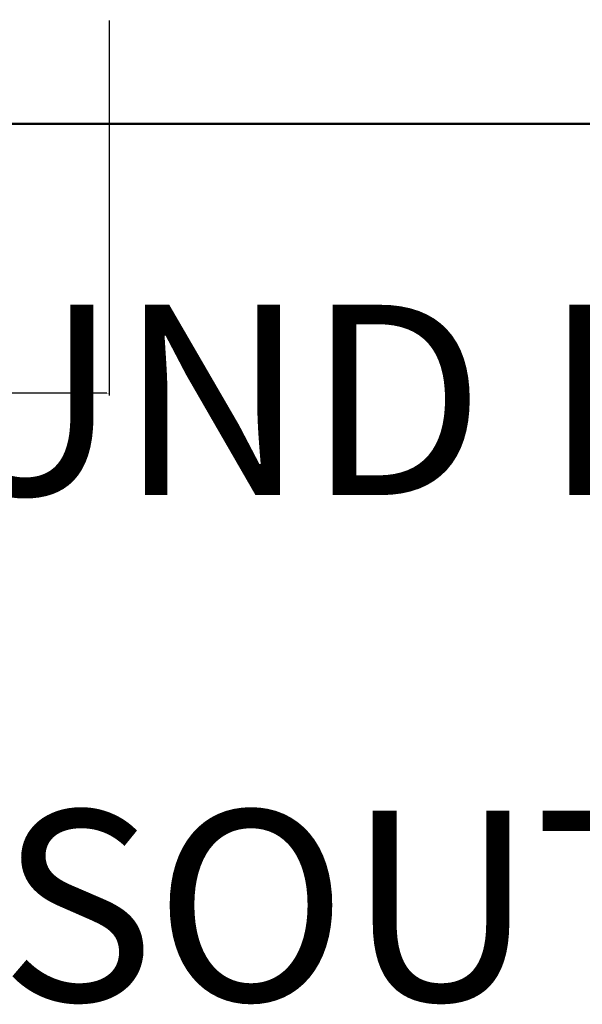
# Model space of a CAD drawing. Units: inches. Extents: x 22042254 to 25404563, y 17568978 to 17626777.
# Tile 24 of 45: x 22179889 to 22179932, y 17626125 to 17626201. Entities that reach past the tile are written whole.
import ezdxf

# ---------------------------------------------------------------- set-up
doc = ezdxf.new("R2010")
doc.units = ezdxf.units.IN
doc.header["$MEASUREMENT"] = 0
for name, color, linetype, lineweight in [('A-ANNO-DIMS', 2, 'Continuous', 18), ('text', 7, 'Continuous', 25), ('walls', 252, 'Continuous', 50)]:
    doc.layers.add(name, color=color, linetype=linetype, lineweight=lineweight)
doc.styles.get("Standard").update_dxf_attribs({"font": 'arial.ttf'})
doc.dimstyles.get("Standard").update_dxf_attribs({"dimtxt": 8, "dimasz": 0.18, "dimexe": 0.18, "dimexo": 0.0625, "dimgap": 0.09, "dimtad": 0, "dimtih": 1, "dimtoh": 1, "dimzin": 0, "dimdsep": 46, "dimlunit": 3, "dimtxsty": 'Standard', "dimcen": 0.09, "dimadec": 0, "dimazin": 0, "dimtfac": 1, "dimtofl": 0, "dimtmove": 0, "dimatfit": 3, "dimfxl": 1, "dimtolj": 1, "dimtzin": 0, "dimarcsym": 0})

# ---------------------------------------------------------------- blocks, each defined once
blk = doc.blocks.new('*D59')
at = {"layer": 'A-ANNO-DIMS', "color": 0, "lineweight": -2, "transparency": 16777216}
for p, q in [((22179802.402, 17626200.497), (22179802.402, 17626171.756)), ((22179895.926, 17626200.497), (22179895.926, 17626171.756)), ((22179802.582, 17626171.936), (22179829.153, 17626171.936)), ((22179895.746, 17626171.936), (22179869.175, 17626171.936))]:
    blk.add_line(p, q, dxfattribs=at)
at = {"layer": 'A-ANNO-DIMS', "color": 0, "transparency": 16777216}
for points in [[(22179802.582, 17626171.966), (22179802.582, 17626171.906), (22179802.402, 17626171.936)], [(22179895.746, 17626171.966), (22179895.746, 17626171.906), (22179895.926, 17626171.936)]]:
    blk.add_solid(points, dxfattribs=at)
at = {"layer": 'Defpoints', "color": 0, "transparency": 16777216}
for p in [(22179802.402, 17626200.559), (22179895.926, 17626200.559), (22179895.926, 17626171.936)]:
    blk.add_point(p, dxfattribs=at)
at = {"layer": 'A-ANNO-DIMS', "color": 0, "transparency": 16777216, "insert": (22179849.164, 17626171.936), "char_height": 8, "attachment_point": 5}
blk.add_mtext('\\A1;7\'-9 1/2"', dxfattribs=at)

msp = doc.modelspace()

# ---------------------------------------------------------------- linework, layer by layer
at = {"layer": 'walls'}
msp.add_line((22179783.734, 17626192.584), (22179936.734, 17626192.584), dxfattribs=at)

# ---------------------------------------------------------------- texts
at = {"layer": 'text'}
for s, p in [('GROUND FLOOR PLAN', (22179841.196, 17626164.124)), ('30X45 SOUTH FACE HOUSE PLAN 3BHK', (22179827.516, 17626125.358))]:
    msp.add_text(s, height=14.58777, dxfattribs=at).set_placement(p)

# ---------------------------------------------------------------- dimensions: what is measured, and where the dimension line sits
at = {"layer": 'A-ANNO-DIMS'}
dim = msp.add_linear_dim(base=(22179895.926, 17626171.936), p1=(22179802.402, 17626200.559), p2=(22179895.926, 17626200.559), dimstyle='Standard', override={"dimdec": 1, "dimlfac": 1, "dimrnd": 0, "dimzin": 1, "dimdsep": 46, "dimlunit": 4, "dimfrac": 2}, dxfattribs=at)
dim.commit()
dim.dimension.update_dxf_attribs({"geometry": '*D59', "text_midpoint": (22179849.164, 17626171.936)})

doc.saveas('drawing.dxf')
